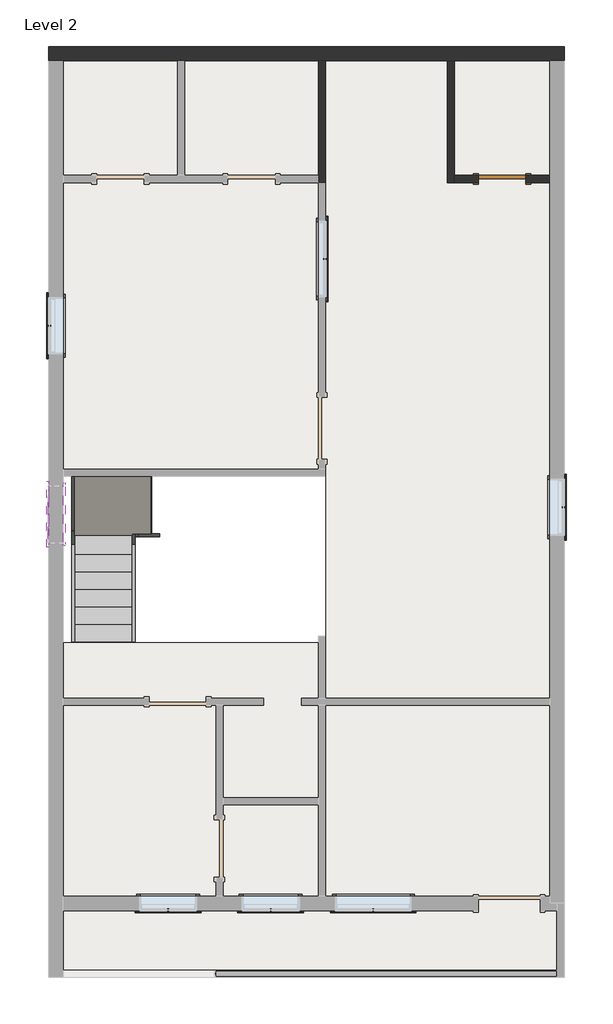
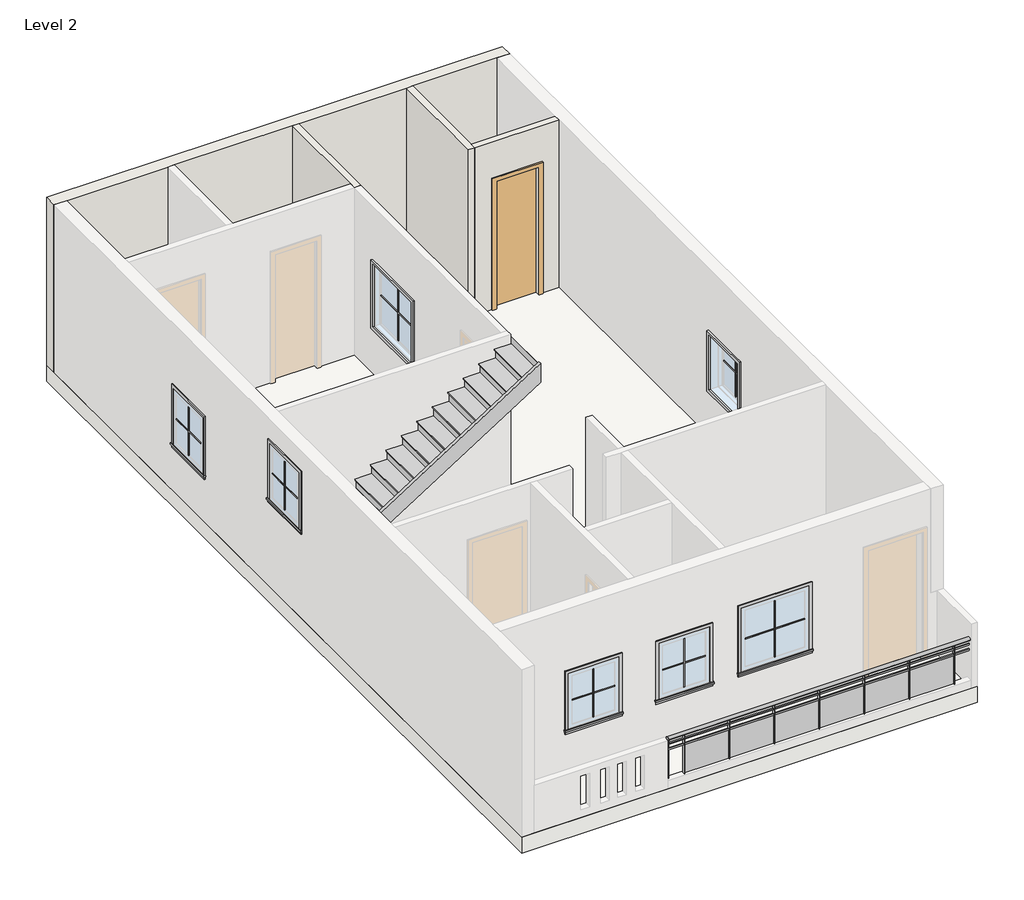
# One storey, part 2 of 2: 21 proxies, 5 members, 4 walls, 2 slabs, 2 stair flights, 1 door, 1 railing.
"""IFC4 building model written with IfcOpenShell, lengths in millimetres."""

from ifc_helpers import new_model, si_unit, point, frame, origin, place, context, project, spatial, polyline, ellipse_curve, trimmed, outline, extrude, faceted_brep, transform, mapped, element, save
from ifc_brep_helpers import plane_surface, extruded_surface, advanced_brep
from components import muntin_pattern_2x2_muntin_pattern_2x2_5e50c346, muntin_pattern_2x2_muntin_pattern_2x2_cef8da4c, muntin_pattern_2x2_muntin_pattern_2x2_8235f178, muntin_pattern_2x2_muntin_pattern_2x2_3e21365d, trim_window_exterior_flat_with_sill_0e7a59f4, trim_window_exterior_flat_with_sill_ac84ebb5, trim_window_exterior_flat_with_sill_7cfdd449, trim_window_exterior_flat_with_sill_1a1a26d5, trim_window_interior_flat_picture_frame_9adb9ca0, trim_window_interior_flat_picture_frame_caf2db4f, trim_window_interior_flat_picture_frame_f1e0b15b, trim_window_interior_flat_picture_frame_dc353545, door_019bc352, non_monolithic_landing_db9d561b, stair_flight_bb85c52a, stair_flight_c36fe085

model = new_model("IFC4")

# Units and contexts
model_context = context("Model", 3, world=origin())
ifc_project = project(units=[si_unit("LENGTHUNIT", "METRE", prefix="MILLI")], contexts=[model_context])

# Site, building, storey
site = spatial("IfcSite", under=ifc_project)
building = spatial("IfcBuilding", under=site)
storey = spatial("IfcBuildingStorey", under=building, Name="Level 2", Elevation=3200.4)

# Proxies
placement = place(None, origin())
muntin_pattern_2x2_muntin_pattern_2x2_shape = muntin_pattern_2x2_muntin_pattern_2x2_5e50c346(model_context)
element("IfcBuildingElementProxy", 1, Name="Muntin Pattern_2x2 : Muntin Pattern_2x2", ObjectType="Muntin Pattern_2x2 : Muntin Pattern_2x2", at=placement, inside=storey, context=model_context, shape_type="MappedRepresentation", body=[
    mapped(muntin_pattern_2x2_muntin_pattern_2x2_shape, transform((-10378.6167709, -3243.6387867, 4184.65), x_axis=(1.0, 0.0, 0.0), y_axis=(0.0, 1.0, 0.0), z_axis=(0.0, 0.0, 1.0))),
])
element("IfcBuildingElementProxy", 2, Name="Muntin Pattern_2x2 : Muntin Pattern_2x2", ObjectType="Muntin Pattern_2x2 : Muntin Pattern_2x2", at=placement, inside=storey, context=model_context, shape_type="MappedRepresentation", body=[
    mapped(muntin_pattern_2x2_muntin_pattern_2x2_shape, transform((-12016.9167709, -3243.6387867, 4184.65), x_axis=(1.0, 0.0, 0.0), y_axis=(0.0, 1.0, 0.0), z_axis=(0.0, 0.0, 1.0))),
])
muntin_pattern_2x2_muntin_pattern_2x2_2_shape = muntin_pattern_2x2_muntin_pattern_2x2_cef8da4c(model_context)
element("IfcBuildingElementProxy", 3, Name="Muntin Pattern_2x2 : Muntin Pattern_2x2", ObjectType="Muntin Pattern_2x2 : Muntin Pattern_2x2", at=placement, inside=storey, context=model_context, shape_type="MappedRepresentation", body=[
    mapped(muntin_pattern_2x2_muntin_pattern_2x2_2_shape, transform((-8740.3167709, -3243.6387867, 4184.65), x_axis=(1.0, 0.0, 0.0), y_axis=(0.0, 1.0, 0.0), z_axis=(0.0, 0.0, 1.0))),
])
muntin_pattern_2x2_muntin_pattern_2x2_3_shape = muntin_pattern_2x2_muntin_pattern_2x2_8235f178(model_context)
element("IfcBuildingElementProxy", 4, Name="Muntin Pattern_2x2 : Muntin Pattern_2x2", ObjectType="Muntin Pattern_2x2 : Muntin Pattern_2x2", at=placement, inside=storey, context=model_context, shape_type="MappedRepresentation", body=[
    mapped(muntin_pattern_2x2_muntin_pattern_2x2_3_shape, transform((-9511.8417709, 7148.1362133, 4184.65), x_axis=(0.0, -1.0, 0.0), y_axis=(1.0, 0.0, 0.0), z_axis=(0.0, 0.0, 1.0))),
])
muntin_pattern_2x2_muntin_pattern_2x2_4_shape = muntin_pattern_2x2_muntin_pattern_2x2_3e21365d(model_context)
element("IfcBuildingElementProxy", 5, Name="Muntin Pattern_2x2 : Muntin Pattern_2x2", ObjectType="Muntin Pattern_2x2 : Muntin Pattern_2x2", at=placement, inside=storey, context=model_context, shape_type="MappedRepresentation", body=[
    mapped(muntin_pattern_2x2_muntin_pattern_2x2_4_shape, transform((-13912.3917709, 6081.3362133, 4184.65), x_axis=(0.0, 1.0, 0.0), y_axis=(-1.0, 0.0, 0.0), z_axis=(0.0, 0.0, 1.0))),
])
element("IfcBuildingElementProxy", 6, Name="Muntin Pattern_2x2 : Muntin Pattern_2x2", ObjectType="Muntin Pattern_2x2 : Muntin Pattern_2x2", at=placement, inside=storey, context=model_context, shape_type="MappedRepresentation", body=[
    mapped(muntin_pattern_2x2_muntin_pattern_2x2_4_shape, transform((-13912.3917709, 3071.4362133, 4964.0778271), x_axis=(0.0, 1.0, 0.0), y_axis=(-1.0, 0.0, 0.0), z_axis=(0.0, 0.0, 1.0))),
])
element("IfcBuildingElementProxy", 7, Name="Muntin Pattern_2x2 : Muntin Pattern_2x2", ObjectType="Muntin Pattern_2x2 : Muntin Pattern_2x2", at=placement, inside=storey, context=model_context, shape_type="MappedRepresentation", body=[
    mapped(muntin_pattern_2x2_muntin_pattern_2x2_4_shape, transform((-5701.8417709, 3185.7362133, 4184.65), x_axis=(0.0, -1.0, 0.0), y_axis=(1.0, 0.0, 0.0), z_axis=(0.0, 0.0, 1.0))),
])
trim_window_exterior_flat_with_sill_shape = trim_window_exterior_flat_with_sill_0e7a59f4(model_context)
element("IfcBuildingElementProxy", 8, Name="Trim-Window-Exterior-Flat : with Sill", ObjectType="Trim-Window-Exterior-Flat : with Sill", at=placement, inside=storey, context=model_context, shape_type="MappedRepresentation", body=[
    mapped(trim_window_exterior_flat_with_sill_shape, transform((-10378.6167709, -3253.1637867, 5181.6), x_axis=(-1.0, 0.0, 0.0), y_axis=(0.0, 0.0, -1.0), z_axis=(0.0, -1.0, 0.0))),
])
element("IfcBuildingElementProxy", 9, Name="Trim-Window-Exterior-Flat : with Sill", ObjectType="Trim-Window-Exterior-Flat : with Sill", at=placement, inside=storey, context=model_context, shape_type="MappedRepresentation", body=[
    mapped(trim_window_exterior_flat_with_sill_shape, transform((-12016.9167709, -3253.1637867, 5181.6), x_axis=(-1.0, 0.0, 0.0), y_axis=(0.0, 0.0, -1.0), z_axis=(0.0, -1.0, 0.0))),
])
trim_window_exterior_flat_with_sill_2_shape = trim_window_exterior_flat_with_sill_ac84ebb5(model_context)
element("IfcBuildingElementProxy", 10, Name="Trim-Window-Exterior-Flat : with Sill", ObjectType="Trim-Window-Exterior-Flat : with Sill", at=placement, inside=storey, context=model_context, shape_type="MappedRepresentation", body=[
    mapped(trim_window_exterior_flat_with_sill_2_shape, transform((-8740.3167709, -3253.1637867, 5334.0), x_axis=(-1.0, 0.0, 0.0), y_axis=(0.0, 0.0, -1.0), z_axis=(0.0, -1.0, 0.0))),
])
trim_window_exterior_flat_with_sill_3_shape = trim_window_exterior_flat_with_sill_7cfdd449(model_context)
element("IfcBuildingElementProxy", 11, Name="Trim-Window-Exterior-Flat : with Sill", ObjectType="Trim-Window-Exterior-Flat : with Sill", at=placement, inside=storey, context=model_context, shape_type="MappedRepresentation", body=[
    mapped(trim_window_exterior_flat_with_sill_3_shape, transform((-9502.3167709, 7148.1362133, 5334.0), x_axis=(0.0, 1.0, 0.0), y_axis=(0.0, 0.0, 1.0), z_axis=(1.0, 0.0, 0.0))),
])
trim_window_exterior_flat_with_sill_4_shape = trim_window_exterior_flat_with_sill_1a1a26d5(model_context)
element("IfcBuildingElementProxy", 12, Name="Trim-Window-Exterior-Flat : with Sill", ObjectType="Trim-Window-Exterior-Flat : with Sill", at=placement, inside=storey, context=model_context, shape_type="MappedRepresentation", body=[
    mapped(trim_window_exterior_flat_with_sill_4_shape, transform((-13921.9167709, 6081.3362133, 5181.6), x_axis=(0.0, -1.0, 0.0), y_axis=(0.0, 0.0, 1.0), z_axis=(-1.0, 0.0, 0.0))),
])
element("IfcBuildingElementProxy", 13, Name="Trim-Window-Exterior-Flat : with Sill", ObjectType="Trim-Window-Exterior-Flat : with Sill", at=placement, inside=storey, context=model_context, shape_type="MappedRepresentation", body=[
    mapped(trim_window_exterior_flat_with_sill_4_shape, transform((-13921.9167709, 3071.4362133, 5961.0278271), x_axis=(0.0, -1.0, 0.0), y_axis=(0.0, 0.0, 1.0), z_axis=(-1.0, 0.0, 0.0))),
])
element("IfcBuildingElementProxy", 14, Name="Trim-Window-Exterior-Flat : with Sill", ObjectType="Trim-Window-Exterior-Flat : with Sill", at=placement, inside=storey, context=model_context, shape_type="MappedRepresentation", body=[
    mapped(trim_window_exterior_flat_with_sill_4_shape, transform((-5692.3167709, 3185.7362133, 5181.6), x_axis=(0.0, 1.0, 0.0), y_axis=(0.0, 0.0, 1.0), z_axis=(1.0, 0.0, 0.0))),
])
trim_window_interior_flat_picture_frame_shape = trim_window_interior_flat_picture_frame_9adb9ca0(model_context)
element("IfcBuildingElementProxy", 15, Name="Trim-Window-Interior-Flat : Picture Frame", ObjectType="Trim-Window-Interior-Flat : Picture Frame", at=placement, inside=storey, context=model_context, shape_type="MappedRepresentation", body=[
    mapped(trim_window_interior_flat_picture_frame_shape, transform((-10378.6167709, -3024.5637867, 5181.6), x_axis=(1.0, 0.0, 0.0), y_axis=(0.0, 0.0, -1.0), z_axis=(0.0, 1.0, 0.0))),
])
element("IfcBuildingElementProxy", 16, Name="Trim-Window-Interior-Flat : Picture Frame", ObjectType="Trim-Window-Interior-Flat : Picture Frame", at=placement, inside=storey, context=model_context, shape_type="MappedRepresentation", body=[
    mapped(trim_window_interior_flat_picture_frame_shape, transform((-12016.9167709, -3024.5637867, 5181.6), x_axis=(1.0, 0.0, 0.0), y_axis=(0.0, 0.0, -1.0), z_axis=(0.0, 1.0, 0.0))),
])
trim_window_interior_flat_picture_frame_2_shape = trim_window_interior_flat_picture_frame_caf2db4f(model_context)
element("IfcBuildingElementProxy", 17, Name="Trim-Window-Interior-Flat : Picture Frame", ObjectType="Trim-Window-Interior-Flat : Picture Frame", at=placement, inside=storey, context=model_context, shape_type="MappedRepresentation", body=[
    mapped(trim_window_interior_flat_picture_frame_2_shape, transform((-8740.3167709, -3024.5637867, 5334.0), x_axis=(1.0, 0.0, 0.0), y_axis=(0.0, 0.0, -1.0), z_axis=(0.0, 1.0, 0.0))),
])
trim_window_interior_flat_picture_frame_3_shape = trim_window_interior_flat_picture_frame_f1e0b15b(model_context)
element("IfcBuildingElementProxy", 18, Name="Trim-Window-Interior-Flat : Picture Frame", ObjectType="Trim-Window-Interior-Flat : Picture Frame", at=placement, inside=storey, context=model_context, shape_type="MappedRepresentation", body=[
    mapped(trim_window_interior_flat_picture_frame_3_shape, transform((-9616.6167709, 7148.1362133, 5334.0), x_axis=(0.0, -1.0, 0.0), y_axis=(0.0, 0.0, 1.0), z_axis=(-1.0, 0.0, 0.0))),
])
trim_window_interior_flat_picture_frame_4_shape = trim_window_interior_flat_picture_frame_dc353545(model_context)
element("IfcBuildingElementProxy", 19, Name="Trim-Window-Interior-Flat : Picture Frame", ObjectType="Trim-Window-Interior-Flat : Picture Frame", at=placement, inside=storey, context=model_context, shape_type="MappedRepresentation", body=[
    mapped(trim_window_interior_flat_picture_frame_4_shape, transform((-13693.3167709, 6081.3362133, 5181.6), x_axis=(0.0, 1.0, 0.0), y_axis=(0.0, 0.0, 1.0), z_axis=(1.0, 0.0, 0.0))),
])
element("IfcBuildingElementProxy", 20, Name="Trim-Window-Interior-Flat : Picture Frame", ObjectType="Trim-Window-Interior-Flat : Picture Frame", at=placement, inside=storey, context=model_context, shape_type="MappedRepresentation", body=[
    mapped(trim_window_interior_flat_picture_frame_4_shape, transform((-13693.3167709, 3071.4362133, 5961.0278271), x_axis=(0.0, 1.0, 0.0), y_axis=(0.0, 0.0, 1.0), z_axis=(1.0, 0.0, 0.0))),
])
element("IfcBuildingElementProxy", 21, Name="Trim-Window-Interior-Flat : Picture Frame", ObjectType="Trim-Window-Interior-Flat : Picture Frame", at=placement, inside=storey, context=model_context, shape_type="MappedRepresentation", body=[
    mapped(trim_window_interior_flat_picture_frame_4_shape, transform((-5920.9167709, 3185.7362133, 5181.6), x_axis=(0.0, -1.0, 0.0), y_axis=(0.0, 0.0, 1.0), z_axis=(-1.0, 0.0, 0.0))),
])

# Door
door_shape = door_019bc352(model_context)
element("IfcDoor", 22, ObjectType="Single-Flush : D3 2'6\" X 7'", at=placement, inside=storey, context=model_context, shape_type="MappedRepresentation", body=[
    mapped(door_shape, transform((-6682.9167709, 8424.4862133, 3200.4), x_axis=(-1.0, 0.0, 0.0), y_axis=(0.0, -1.0, 0.0), z_axis=(0.0, 0.0, 1.0))),
])

# Members
element("IfcMember", 23, ObjectType="Stringer - 2\" Width", at=placement, inside=storey, context=model_context, shape_type="SweptSolid", body=[
    extrude(outline(polyline([(1037.2129676, 3200.4), (1037.2129676, 3415.4106437), (2774.881956, 4521.2), (2863.6399255, 4216.4), (1267.0684969, 3200.4), (1037.2129676, 3200.4)])), frame((-13559.5954771, 0.0, 0.0), z_axis=(1.0, 0.0, 0.0), x_axis=(0.0, 1.0, 0.0)), (0.0, 0.0, 1.0), 50.8),
])
element("IfcMember", 24, ObjectType="Stringer - 2\" Width", at=placement, inside=storey, context=model_context, shape_type="SweptSolid", body=[
    extrude(outline(polyline([(1037.2129676, 3200.4), (1037.2129676, 3415.4106437), (2764.4129676, 4514.5379164), (2764.4129676, 4153.2555722), (1267.0684969, 3200.4), (1037.2129676, 3200.4)])), frame((-12594.3954771, 0.0, 0.0), z_axis=(1.0, 0.0, 0.0), x_axis=(0.0, 1.0, 0.0)), (0.0, 0.0, 1.0), 50.8),
])
element("IfcMember", 25, ObjectType="Stringer - 2\" Width", at=placement, inside=storey, context=model_context, shape_type="SweptSolid", body=[
    extrude(outline(polyline([(4521.2, -12533.1264887), (4216.4, -12444.3685192), (6076.7282995, -9520.9954771), (6438.0106437, -9520.9954771), (4521.2, -12533.1264887)])), frame((0.0, 2713.6129676, 0.0), z_axis=(0.0, 1.0, 0.0), x_axis=(0.0, 0.0, 1.0)), (0.0, 0.0, 1.0), 50.8),
])
element("IfcMember", 26, ObjectType="Stringer - 2\" Width", at=placement, inside=storey, context=model_context, shape_type="SweptSolid", body=[
    extrude(outline(polyline([(3678.8129676, 4521.2), (3678.8129676, 4216.4), (2863.6399255, 4216.4), (2774.881956, 4521.2), (3678.8129676, 4521.2)])), frame((-13559.5954771, 0.0, 0.0), z_axis=(1.0, 0.0, 0.0), x_axis=(0.0, 1.0, 0.0)), (0.0, 0.0, 1.0), 50.8),
])
element("IfcMember", 27, ObjectType="Stringer - 2\" Width", at=placement, inside=storey, context=model_context, shape_type="SweptSolid", body=[
    extrude(outline(polyline([(4521.2, -12543.5954771), (4216.4, -12543.5954771), (4216.4, -12444.3685192), (4521.2, -12533.1264887), (4521.2, -12543.5954771)])), frame((0.0, 2713.6129676, 0.0), z_axis=(0.0, 1.0, 0.0), x_axis=(0.0, 0.0, 1.0)), (0.0, 0.0, 1.0), 50.8),
])

# Railing
element("IfcRailing", 28, ObjectType="Glass Panel - Bottom Fill", at=placement, inside=storey, context=model_context, shape_type="SolidModel", body=[
    advanced_brep(
    [(-11254.9167709, -4224.7137867, 4114.8), (-11254.9167709, -4300.9137867, 4114.8), (-5793.9167709, -4224.7137867, 4114.8), (-5793.9167709, -4300.9137867, 4114.8)],
    [
        (0, 1, ellipse_curve(frame((-11254.9167709, -4262.8137867, 4114.8), z_axis=(-1.0, 0.0, 0.0), x_axis=(0.0, -1.0, 0.0)), 38.1, 28.575)),
        (1, 0, ellipse_curve(frame((-11254.9167709, -4262.8137867, 4114.8), z_axis=(-1.0, 0.0, 0.0), x_axis=(0.0, -1.0, 0.0)), 38.1, 28.575)),
        (2, 3, ellipse_curve(frame((-5793.9167709, -4262.8137867, 4114.8), z_axis=(1.0, 0.0, 0.0), x_axis=(0.0, -1.0, 0.0)), 38.1, 28.575)),
        (3, 2, ellipse_curve(frame((-5793.9167709, -4262.8137867, 4114.8), z_axis=(1.0, 0.0, 0.0), x_axis=(0.0, -1.0, 0.0)), 38.1, 28.575)),
        (0, 2),
        (3, 1),
    ],
    [
        plane_surface(frame((-11254.9167709, -4262.8137867, 4114.8), z_axis=(-1.0, 0.0, 0.0), x_axis=(0.0, 1.0, 0.0))),
        plane_surface(frame((-5793.9167709, -4262.8137867, 4114.8), z_axis=(1.0, 0.0, 0.0), x_axis=(0.0, 1.0, 0.0))),
        extruded_surface(trimmed(ellipse_curve(frame((-5793.9167709, -4262.8137867, 4114.8), z_axis=(-1.0, 0.0, 0.0), x_axis=(0.0, -1.0, 0.0)), 38.1, 28.575), [point((-5793.9167709, -4224.7137867, 4114.8))], [point((-5793.9167709, -4300.9137867, 4114.8))], True, "CARTESIAN"), (-5460.999999999999, 0.0, 0.0), 5460.999999999999),
        extruded_surface(trimmed(ellipse_curve(frame((-5793.9167709, -4262.8137867, 4114.8), z_axis=(-1.0, 0.0, 0.0), x_axis=(0.0, -1.0, 0.0)), 38.1, 28.575), [point((-5793.9167709, -4300.9137867, 4114.8))], [point((-5793.9167709, -4224.7137867, 4114.8))], True, "CARTESIAN"), (-5460.999999999999, 0.0, 0.0), 5460.999999999999),
    ],
    [
        (0, [[1, 2]]),
        (1, [[3, 4]]),
        (2, [[-1, 5, -4, 6]]),
        (3, [[-2, -6, -3, -5]]),
    ],
),
    extrude(outline(polyline([(-11254.9167709, -4275.5137867), (-11254.9167709, -4250.1137867), (-5793.9167709, -4250.1137867), (-5793.9167709, -4275.5137867), (-11254.9167709, -4275.5137867)])), frame((0.0, 0.0, 4000.5), z_axis=(0.0, 0.0, 1.0), x_axis=(1.0, 0.0, 0.0)), (0.0, 0.0, 1.0), 25.4),
    extrude(outline(polyline([(-11254.9167709, -4275.5137867), (-11254.9167709, -4250.1137867), (-5793.9167709, -4250.1137867), (-5793.9167709, -4275.5137867), (-11254.9167709, -4275.5137867)])), frame((0.0, 0.0, 3898.9), z_axis=(0.0, 0.0, 1.0), x_axis=(1.0, 0.0, 0.0)), (0.0, 0.0, 1.0), 25.4),
    extrude(outline(polyline([(-6092.3667709, -4288.2137867), (-6092.3667709, -4237.4137867), (-6079.6667709, -4237.4137867), (-6079.6667709, -4288.2137867), (-6092.3667709, -4288.2137867)])), frame((0.0, 0.0, 3200.4), z_axis=(0.0, 0.0, 1.0), x_axis=(1.0, 0.0, 0.0)), (0.0, 0.0, 1.0), 885.825),
    extrude(outline(polyline([(-6898.8167709, -4256.2786297), (-6086.0167709, -4256.2786297), (-6086.0167709, -4262.6286297), (-6898.8167709, -4262.6286297), (-6898.8167709, -4256.2786297)])), frame((0.0, 0.0, 3302.0), z_axis=(0.0, 0.0, 1.0), x_axis=(1.0, 0.0, 0.0)), (0.0, 0.0, 1.0), 596.9),
    extrude(outline(polyline([(-6905.1667709, -4288.2137867), (-6905.1667709, -4237.4137867), (-6892.4667709, -4237.4137867), (-6892.4667709, -4288.2137867), (-6905.1667709, -4288.2137867)])), frame((0.0, 0.0, 3200.4), z_axis=(0.0, 0.0, 1.0), x_axis=(1.0, 0.0, 0.0)), (0.0, 0.0, 1.0), 885.825),
    extrude(outline(polyline([(-7711.6167709, -4256.2786297), (-6898.8167709, -4256.2786297), (-6898.8167709, -4262.6286297), (-7711.6167709, -4262.6286297), (-7711.6167709, -4256.2786297)])), frame((0.0, 0.0, 3302.0), z_axis=(0.0, 0.0, 1.0), x_axis=(1.0, 0.0, 0.0)), (0.0, 0.0, 1.0), 596.9),
    extrude(outline(polyline([(-7717.9667709, -4288.2137867), (-7717.9667709, -4237.4137867), (-7705.2667709, -4237.4137867), (-7705.2667709, -4288.2137867), (-7717.9667709, -4288.2137867)])), frame((0.0, 0.0, 3200.4), z_axis=(0.0, 0.0, 1.0), x_axis=(1.0, 0.0, 0.0)), (0.0, 0.0, 1.0), 885.825),
    extrude(outline(polyline([(-8524.4167709, -4256.2786297), (-7711.6167709, -4256.2786297), (-7711.6167709, -4262.6286297), (-8524.4167709, -4262.6286297), (-8524.4167709, -4256.2786297)])), frame((0.0, 0.0, 3302.0), z_axis=(0.0, 0.0, 1.0), x_axis=(1.0, 0.0, 0.0)), (0.0, 0.0, 1.0), 596.9),
    extrude(outline(polyline([(-8530.7667709, -4288.2137867), (-8530.7667709, -4237.4137867), (-8518.0667709, -4237.4137867), (-8518.0667709, -4288.2137867), (-8530.7667709, -4288.2137867)])), frame((0.0, 0.0, 3200.4), z_axis=(0.0, 0.0, 1.0), x_axis=(1.0, 0.0, 0.0)), (0.0, 0.0, 1.0), 885.825),
    extrude(outline(polyline([(-9337.2167709, -4256.2786297), (-8524.4167709, -4256.2786297), (-8524.4167709, -4262.6286297), (-9337.2167709, -4262.6286297), (-9337.2167709, -4256.2786297)])), frame((0.0, 0.0, 3302.0), z_axis=(0.0, 0.0, 1.0), x_axis=(1.0, 0.0, 0.0)), (0.0, 0.0, 1.0), 596.9),
    extrude(outline(polyline([(-9343.5667709, -4288.2137867), (-9343.5667709, -4237.4137867), (-9330.8667709, -4237.4137867), (-9330.8667709, -4288.2137867), (-9343.5667709, -4288.2137867)])), frame((0.0, 0.0, 3200.4), z_axis=(0.0, 0.0, 1.0), x_axis=(1.0, 0.0, 0.0)), (0.0, 0.0, 1.0), 885.825),
    extrude(outline(polyline([(-10150.0167709, -4256.2786297), (-9337.2167709, -4256.2786297), (-9337.2167709, -4262.6286297), (-10150.0167709, -4262.6286297), (-10150.0167709, -4256.2786297)])), frame((0.0, 0.0, 3302.0), z_axis=(0.0, 0.0, 1.0), x_axis=(1.0, 0.0, 0.0)), (0.0, 0.0, 1.0), 596.9),
    extrude(outline(polyline([(-10156.3667709, -4288.2137867), (-10156.3667709, -4237.4137867), (-10143.6667709, -4237.4137867), (-10143.6667709, -4288.2137867), (-10156.3667709, -4288.2137867)])), frame((0.0, 0.0, 3200.4), z_axis=(0.0, 0.0, 1.0), x_axis=(1.0, 0.0, 0.0)), (0.0, 0.0, 1.0), 885.825),
    extrude(outline(polyline([(-10962.8167709, -4256.2786297), (-10150.0167709, -4256.2786297), (-10150.0167709, -4262.6286297), (-10962.8167709, -4262.6286297), (-10962.8167709, -4256.2786297)])), frame((0.0, 0.0, 3302.0), z_axis=(0.0, 0.0, 1.0), x_axis=(1.0, 0.0, 0.0)), (0.0, 0.0, 1.0), 596.9),
    extrude(outline(polyline([(-10969.1667709, -4288.2137867), (-10969.1667709, -4237.4137867), (-10956.4667709, -4237.4137867), (-10956.4667709, -4288.2137867), (-10969.1667709, -4288.2137867)])), frame((0.0, 0.0, 3200.4), z_axis=(0.0, 0.0, 1.0), x_axis=(1.0, 0.0, 0.0)), (0.0, 0.0, 1.0), 885.825),
    extrude(outline(polyline([(-5806.6167709, -4272.3387867), (-5806.6167709, -4253.2887867), (-5787.5667709, -4253.2887867), (-5787.5667709, -4272.3387867), (-5806.6167709, -4272.3387867)])), frame((0.0, 0.0, 3200.4), z_axis=(0.0, 0.0, 1.0), x_axis=(1.0, 0.0, 0.0)), (0.0, 0.0, 1.0), 885.825),
    extrude(outline(polyline([(-11261.2667709, -4272.3387867), (-11261.2667709, -4253.2887867), (-11242.2167709, -4253.2887867), (-11242.2167709, -4272.3387867), (-11261.2667709, -4272.3387867)])), frame((0.0, 0.0, 3200.4), z_axis=(0.0, 0.0, 1.0), x_axis=(1.0, 0.0, 0.0)), (0.0, 0.0, 1.0), 885.825),
])

# Slabs
element("IfcSlab", 29, ObjectType="Generic - 12\"", at=placement, inside=storey, context=model_context, shape_type="SweptSolid", body=[
    extrude(outline(polyline([(-5692.3167709, 10539.0362133), (-5692.3167709, -4319.9637867), (-13921.9167709, -4319.9637867), (-13921.9167709, 10539.0362133), (-5692.3167709, 10539.0362133)]), holes=[polyline([(-9502.3167709, 3681.0362133), (-13693.3167709, 3681.0362133), (-13693.3167709, 1031.225127), (-9502.3167709, 1031.225127), (-9502.3167709, 3681.0362133)])]), frame((0.0, 0.0, 2895.6), z_axis=(0.0, 0.0, 1.0), x_axis=(1.0, 0.0, 0.0)), (0.0, 0.0, 1.0), 304.8),
])
non_monolithic_landing_shape = non_monolithic_landing_db9d561b(model_context)
element("IfcSlab", 30, ObjectType="Non-Monolithic Landing", at=placement, inside=storey, context=model_context, shape_type="MappedRepresentation", body=[
    mapped(non_monolithic_landing_shape, transform((0.0, 0.0, 0.0), x_axis=(1.0, 0.0, 0.0), y_axis=(0.0, 1.0, 0.0), z_axis=(0.0, 0.0, 1.0))),
])

# Stair flights
stair_flight_shape = stair_flight_bb85c52a(model_context)
element("IfcStairFlight", 31, ObjectType="2\" Tread 1\" Nosing 1/4\" Riser", at=placement, inside=storey, context=model_context, shape_type="MappedRepresentation", body=[
    mapped(stair_flight_shape, transform((0.0, 0.0, 0.0), x_axis=(1.0, 0.0, 0.0), y_axis=(0.0, 1.0, 0.0), z_axis=(0.0, 0.0, 1.0))),
])
stair_flight_2_shape = stair_flight_c36fe085(model_context)
element("IfcStairFlight", 32, ObjectType="2\" Tread 1\" Nosing 1/4\" Riser", at=placement, inside=storey, context=model_context, shape_type="MappedRepresentation", body=[
    mapped(stair_flight_2_shape, transform((0.0, 0.0, 0.0), x_axis=(1.0, 0.0, 0.0), y_axis=(0.0, 1.0, 0.0), z_axis=(0.0, 0.0, 1.0))),
])

# Walls
element("IfcWall", 33, ObjectType="4.5\" inner wall", at=placement, inside=storey, context=model_context, shape_type="Brep", body=[
    faceted_brep([(-9616.6167709, 10310.4362133, 3200.4), (-9616.6167709, 8481.6362133, 3200.4), (-9616.6167709, 8367.3362133, 3200.4), (-9616.6167709, 8367.3362133, 6400.8), (-9616.6167709, 8481.6362133, 6400.8), (-9616.6167709, 10310.4362133, 6400.8), (-9502.3167709, 10310.4362133, 3200.4), (-9502.3167709, 10310.4362133, 6400.8), (-9502.3167709, 8367.3362133, 6400.8), (-9502.3167709, 8367.3362133, 3200.4)], [[[0, 1, 2, 3, 4, 5]], [[6, 7, 8, 9]], [[2, 1, 0, 6, 9]], [[5, 4, 3, 8, 7]], [[0, 5, 7, 6]], [[3, 2, 9, 8]]]),
])
element("IfcWall", 34, ObjectType="4.5\" inner wall", at=placement, inside=storey, context=model_context, shape_type="Brep", body=[
    faceted_brep([(-7559.2167709, 10310.4362133, 3200.4), (-7559.2167709, 8367.3362133, 3200.4), (-7559.2167709, 8367.3362133, 6400.8), (-7559.2167709, 10310.4362133, 6400.8), (-7444.9167709, 10310.4362133, 3200.4), (-7444.9167709, 10310.4362133, 6400.8), (-7444.9167709, 8481.6362133, 6400.8), (-7444.9167709, 8367.3362133, 6400.8), (-7444.9167709, 8367.3362133, 3200.4), (-7444.9167709, 8481.6362133, 3200.4)], [[[0, 1, 2, 3]], [[4, 5, 6, 7, 8, 9]], [[1, 0, 4, 9, 8]], [[3, 2, 7, 6, 5]], [[0, 3, 5, 4]], [[2, 1, 8, 7]]]),
])
element("IfcWall", 35, ObjectType="4.5\" inner wall", at=placement, inside=storey, context=model_context, shape_type="SweptSolid", body=[
    extrude(outline(polyline([(3200.4, -7444.9167709), (3200.4, -7063.9167709), (5638.8, -7063.9167709), (5638.8, -6301.9167709), (3200.4, -6301.9167709), (3200.4, -5920.9167709), (6400.8, -5920.9167709), (6400.8, -7444.9167709), (3200.4, -7444.9167709)])), frame((0.0, 8367.3362133, 0.0), z_axis=(0.0, 1.0, 0.0), x_axis=(0.0, 0.0, 1.0)), (0.0, 0.0, 1.0), 114.3),
])
element("IfcWall", 36, ObjectType="9\" outer wall", at=placement, inside=storey, context=model_context, shape_type="Brep", body=[
    faceted_brep([(-13921.9167709, 10310.4362133, 3200.4), (-13693.3167709, 10310.4362133, 3200.4), (-11864.5167709, 10310.4362133, 3200.4), (-11750.2167709, 10310.4362133, 3200.4), (-9616.6167709, 10310.4362133, 3200.4), (-9502.3167709, 10310.4362133, 3200.4), (-7559.2167709, 10310.4362133, 3200.4), (-7444.9167709, 10310.4362133, 3200.4), (-5920.9167709, 10310.4362133, 3200.4), (-5692.3167709, 10310.4362133, 3200.4), (-5692.3167709, 10310.4362133, 6400.8), (-5920.9167709, 10310.4362133, 6400.8), (-7444.9167709, 10310.4362133, 6400.8), (-7559.2167709, 10310.4362133, 6400.8), (-9502.3167709, 10310.4362133, 6400.8), (-9616.6167709, 10310.4362133, 6400.8), (-11750.2167709, 10310.4362133, 6400.8), (-11864.5167709, 10310.4362133, 6400.8), (-13693.3167709, 10310.4362133, 6400.8), (-13921.9167709, 10310.4362133, 6400.8), (-13921.9167709, 10539.0362133, 3200.4), (-13921.9167709, 10539.0362133, 6400.8), (-5692.3167709, 10539.0362133, 6400.8), (-5692.3167709, 10539.0362133, 3200.4)], [[[0, 1, 2, 3, 4, 5, 6, 7, 8, 9, 10, 11, 12, 13, 14, 15, 16, 17, 18, 19]], [[20, 21, 22, 23]], [[9, 8, 7, 6, 5, 4, 3, 2, 1, 0, 20, 23]], [[19, 18, 17, 16, 15, 14, 13, 12, 11, 10, 22, 21]], [[10, 9, 23, 22]], [[0, 19, 21, 20]]]),
])

save(model, "model.ifc")

# Revit data of these elements
# Type "Muntin Pattern_2x2 : Muntin Pattern_2x2"
#   Width [instance default] = 4' - 0"
#   Thickness = 0' - 0 1/2"
#   Height [instance default] = 4' - 0"
#   Distance = 0' - 0 3/4"
#   Interior Material [instance default] = none
#   Exterior Material [instance default] = none
#   Default Elevation = 0
# Type "Trim-Window-Exterior-Flat : with Sill"
#   Trim Width = 0' - 2 1/4"
#   Trim Thickness_Picture Frame = 0' - 1 1/4"
#   Trim Thickness_with Sill = 0' - 0 3/4"
#   Sill Thickness = 0' - 1 1/4"
#   Opening Width [instance default] = 2' - 0"
#   Opening Height [instance default] = 3' - 0"
#   Default Elevation = 4' - 0"
#   Sill = yes
#   Picture Frame = no
#   Trim Material [instance default] = none
# Type "Trim-Window-Interior-Flat : Picture Frame"
#   Trim Thickness_Picture Frame = 0' - 1 1/4"
#   Trim Width = 0' - 2 1/4"
#   Trim Thickness_with Sill = 0' - 0 3/4"
#   Sill Thickness = 0' - 1 1/4"
#   Opening Width [instance default] = 2' - 0"
#   Opening Height [instance default] = 3' - 0"
#   Default Elevation = 4' - 0"
#   Sill = no
#   Picture Frame = yes
#   Trim Material [instance default] = none
# Type "Single-Flush : D3 2'6\" X 7'"
#   Type Mark = "11"
#   Construction Type Id = "MDOOR"
#   Assembly Code = "C1020"
#   Analytic Construction = "Metal"
#   Thickness = 0' - 2"
#   Heat Transfer Coefficient (U) = 0.651978 BTU/(h·ft²·°F)
#   Height = 8' - 0"
#   Trim Projection Ext = 0' - 1"
#   Trim Projection Int = 0' - 1"
#   Trim Width = 0' - 3"
#   Width = 2' - 6"
#   Define Thermal Properties by = 1
#   Door Material = Door - Panel
#   Frame Material = Door - Frame
#   Visual Light Transmittance = 0
#   Solar Heat Gain Coefficient = 0
#   Function = (empty or 0)
#   Wall Closure = (empty or 0)
# Type "Glass Panel - Bottom Fill"
#   Assembly Code = "C2010400"
#   built-in parameter 1008612 = 0.0416667 (stored number, unit not read)
#   built-in parameter 1008611 = 0.0416667 (stored number, unit not read)
#   built-in parameter 1008609 = 0.333333 (stored number, unit not read)
#   built-in parameter 1008604 = 0.166667 (stored number, unit not read)
#   built-in parameter 1008603 = 0.166667 (stored number, unit not read)
#   Railing Height = 3' - 0"
#   built-in parameter 1008630 = 2
#   built-in parameter 1008610 = 2
#   built-in parameter 1008618 = Baluster - Square : 3/4"
# Type "Generic - 12\""
#   Assembly Code = "B1010"
#   Function = 0
#   Layers, outside or top first: 1' - 0" no material (function 1)
# Type "4.5\" inner wall"
#   Assembly Code = "B2010"
#   Layers, outside or top first: 0' - 4 1/2" no material (function 1)
# Type "9\" outer wall"
#   Assembly Code = "B2010"
#   Layers, outside or top first: 0' - 9" no material (function 1)
# Elements 1, 2, 5, 6, 7 (IfcBuildingElementProxy, "Muntin Pattern_2x2 : Muntin Pattern_2x2")
#   Width = 2' - 6 1/2"
#   Height = 3' - 0 1/2"
#   Interior Material = Wood - Stained
#   Exterior Material = Clad - White
#   Phase Created = New Construction
#   Materials on its faces: "Clad - White", "Wood - Stained"
# Elements 3, 4 (IfcBuildingElementProxy, "Muntin Pattern_2x2 : Muntin Pattern_2x2")
#   Width = 3' - 6 1/2"
#   Height = 3' - 6 1/2"
#   Interior Material = Wood - Stained
#   Exterior Material = Clad - White
#   Phase Created = New Construction
#   Materials on its faces: "Clad - White", "Wood - Stained"
# Elements 8, 9, 12, 13, 14 (IfcBuildingElementProxy, "Trim-Window-Exterior-Flat : with Sill")
#   Opening Width = 3' - 0"
#   Opening Height = 3' - 6"
#   Trim Material = Clad - White
#   Phase Created = New Construction
#   Materials on its faces: "Clad - White"
# Elements 10, 11 (IfcBuildingElementProxy, "Trim-Window-Exterior-Flat : with Sill")
#   Opening Width = 4' - 0"
#   Opening Height = 4' - 0"
#   Trim Material = Clad - White
#   Phase Created = New Construction
#   Materials on its faces: "Clad - White"
# Elements 15, 16, 19, 20, 21 (IfcBuildingElementProxy, "Trim-Window-Interior-Flat : Picture Frame")
#   Opening Width = 3' - 0"
#   Opening Height = 3' - 6"
#   Trim Material = Wood - Stained
#   Phase Created = New Construction
#   Materials on its faces: "Wood - Stained"
# Elements 17, 18 (IfcBuildingElementProxy, "Trim-Window-Interior-Flat : Picture Frame")
#   Opening Width = 4' - 0"
#   Opening Height = 4' - 0"
#   Trim Material = Wood - Stained
#   Phase Created = New Construction
#   Materials on its faces: "Wood - Stained"
# Element 22 (IfcDoor, "Single-Flush : D3 2'6\" X 7'")
#   Phase Created = New Construction
#   Materials on its faces: "Door - Frame", "Door - Panel"
# Elements 23, 24, 25, 26, 27 (IfcMember, "Stringer - 2\" Width")
#   Phase Created = New Construction
# Element 28 (IfcRailing, "Glass Panel - Bottom Fill")
#   Phase Created = New Construction
#   Materials on its faces: "Glass"
# Element 29 (IfcSlab, "Generic - 12\"")
#   Height Offset From Level = 0' - 0"
#   Phase Created = New Construction
#   Materials on its faces: "Default Floor"
# Element 30 (IfcSlab, "Non-Monolithic Landing")
#   Phase Created = New Construction
# Elements 31, 32 (IfcStairFlight, "2\" Tread 1\" Nosing 1/4\" Riser")
#   Phase Created = New Construction
# Elements 33, 34, 35 (IfcWall, "4.5\" inner wall")
#   Top Offset = 0' - 0"
#   Base Offset = 0' - 0"
#   wall height = 10' - 6"
#   Phase Created = New Construction
#   Base Constraint = Level 2
#   Top Constraint = Level 3
#   Materials on its faces: "Default Wall"
# Element 36 (IfcWall, "9\" outer wall")
#   Top Offset = 0' - 0"
#   Base Offset = 0' - 0"
#   wall height = 10' - 6"
#   Phase Created = New Construction
#   Base Constraint = Level 2
#   Top Constraint = Level 3
#   Materials on its faces: "Default Wall"
# Materials
#   "Door - Panel": class "Wood", colour RGB 210 159 95, transparency 0, Cost = 0
#   "Door - Frame": colour RGB 118 70 51, transparency 0, Cost = 0
#   "Clad - White": class "Wood", colour RGB 242 242 238, transparency 0, Cost = 0
#   "Wood - Stained": class "Wood", colour RGB 224 178 126, transparency 0, Cost = 0
#   "Glass": class "Glass", colour RGB 0 128 192, transparency 0.75, Description = "Soda Lime Glass", Cost = 0
#   "Default Floor": colour RGB 128 128 128, transparency 0, Cost = 0
#   "Default Wall": colour RGB 128 128 128, transparency 0, Cost = 0
